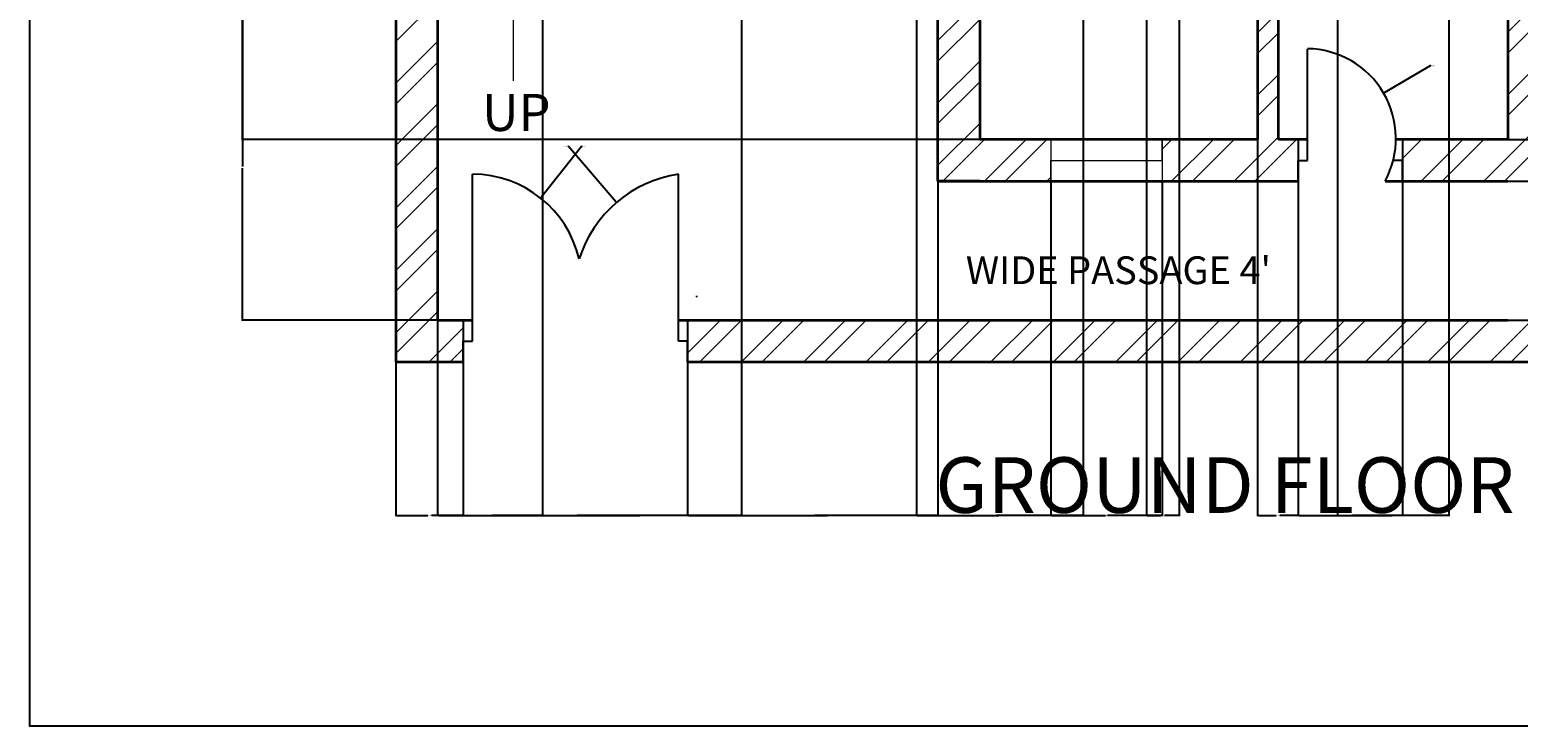
# Model space of a CAD drawing. Units: inches. Extents: x 1595 to 2135, y 460 to 2061.
# Tile 1 of 5: x 1595 to 1917, y 1320 to 1470. Entities that reach past the tile are written whole.
import ezdxf

# ---------------------------------------------------------------- set-up
doc = ezdxf.new("R2010")
doc.units = ezdxf.units.IN
for name, color, linetype, lineweight in [('A-ANNO-DIMS', 2, 'Continuous', 18), ('A-ANNO-SYMB', 7, 'Continuous', 18), ('A-ANNO-TTLB', 7, 'Continuous', 25), ('A-AREA-IDEN', 7, 'Continuous', 18), ('A-DOOR', 3, 'Continuous', 25), ('A-GLAZ', 4, 'Continuous', 18), ('A-WALL', 7, 'Continuous', 35)]:
    doc.layers.add(name, color=color, linetype=linetype, lineweight=lineweight)
doc.layers.add('A-WALL-PATT', color=143, linetype='Continuous', lineweight=13, true_color=0x7aafdf)
doc.styles.get("Standard").update_dxf_attribs({"font": 'arial.ttf'})
doc.dimstyles.get("Standard").update_dxf_attribs({"dimtxt": 0.18, "dimasz": 0.18, "dimexe": 0.18, "dimexo": 0.0625, "dimgap": 0.09, "dimtad": 0, "dimtih": 1, "dimtoh": 1, "dimdec": 4, "dimzin": 0, "dimdsep": 46, "dimtxsty": 'Standard', "dimcen": 0.09, "dimadec": 0, "dimazin": 0, "dimtfac": 1, "dimtdec": 4, "dimtofl": 0, "dimtmove": 0, "dimatfit": 3, "dimfxl": 1, "dimtolj": 1, "dimtzin": 0, "dimarcsym": 0})

# ---------------------------------------------------------------- blocks, each defined once
blk = doc.blocks.new('*D8')
at = {"layer": 'A-ANNO-DIMS', "color": 0, "lineweight": -2, "transparency": 16777216}
for p, q in [((1674.31, 1398.58), (1674.31, 1365.31)), ((1688.85, 1398.58), (1688.85, 1365.31)), ((1674.49, 1365.49), (1681.2, 1365.49)), ((1688.67, 1365.49), (1681.97, 1365.49))]:
    blk.add_line(p, q, dxfattribs=at)
at = {"layer": 'A-ANNO-DIMS', "color": 0, "transparency": 16777216}
for points in [[(1674.49, 1365.52), (1674.49, 1365.46), (1674.31, 1365.49)], [(1688.67, 1365.52), (1688.67, 1365.46), (1688.85, 1365.49)]]:
    blk.add_solid(points, dxfattribs=at)
at = {"layer": 'Defpoints', "color": 0, "transparency": 16777216}
for p in [(1674.31, 1398.64), (1688.85, 1398.64), (1688.85, 1365.49)]:
    blk.add_point(p, dxfattribs=at)
at = {"layer": 'A-ANNO-DIMS', "color": 0, "transparency": 16777216, "insert": (1681.58, 1365.49), "char_height": 0.18, "attachment_point": 5}
blk.add_mtext('\\A1;14.54', dxfattribs=at)
blk = doc.blocks.new('*D9')
at = {"layer": 'A-ANNO-DIMS', "color": 0, "lineweight": -2, "transparency": 16777216}
for p, q in [((1688.85, 1398.58), (1688.85, 1365.31)), ((1737.28, 1398.58), (1737.28, 1365.31)), ((1689.03, 1365.49), (1712.67, 1365.49)), ((1737.1, 1365.49), (1713.46, 1365.49))]:
    blk.add_line(p, q, dxfattribs=at)
at = {"layer": 'A-ANNO-DIMS', "color": 0, "transparency": 16777216}
for points in [[(1689.03, 1365.52), (1689.03, 1365.46), (1688.85, 1365.49)], [(1737.1, 1365.52), (1737.1, 1365.46), (1737.28, 1365.49)]]:
    blk.add_solid(points, dxfattribs=at)
at = {"layer": 'Defpoints', "color": 0, "transparency": 16777216}
for p in [(1688.85, 1398.64), (1737.28, 1398.64), (1737.28, 1365.49)]:
    blk.add_point(p, dxfattribs=at)
at = {"layer": 'A-ANNO-DIMS', "color": 0, "transparency": 16777216, "insert": (1713.06, 1365.49), "char_height": 0.18, "attachment_point": 5}
blk.add_mtext('\\A1;48.42', dxfattribs=at)
blk = doc.blocks.new('*D10')
at = {"layer": 'A-ANNO-DIMS', "color": 0, "lineweight": -2, "transparency": 16777216}
for p, q in [((1791.31, 1437.58), (1791.31, 1365.31)), ((1737.28, 1398.58), (1737.28, 1365.31)), ((1737.46, 1365.49), (1763.9, 1365.49)), ((1791.13, 1365.49), (1764.69, 1365.49))]:
    blk.add_line(p, q, dxfattribs=at)
at = {"layer": 'A-ANNO-DIMS', "color": 0, "transparency": 16777216}
for points in [[(1737.46, 1365.52), (1737.46, 1365.46), (1737.28, 1365.49)], [(1791.13, 1365.52), (1791.13, 1365.46), (1791.31, 1365.49)]]:
    blk.add_solid(points, dxfattribs=at)
at = {"layer": 'Defpoints', "color": 0, "transparency": 16777216}
for p in [(1791.31, 1437.64), (1737.28, 1398.64), (1791.31, 1365.49)]:
    blk.add_point(p, dxfattribs=at)
at = {"layer": 'A-ANNO-DIMS', "color": 0, "transparency": 16777216, "insert": (1764.29, 1365.49), "char_height": 0.18, "attachment_point": 5}
blk.add_mtext('\\A1;54.04', dxfattribs=at)
blk = doc.blocks.new('*D23')
at = {"layer": 'A-ANNO-DIMS', "color": 0, "lineweight": -2, "transparency": 16777216}
for p, q in [((1683.31, 1938.58), (1683.31, 1365.31)), ((1705.98, 1938.58), (1705.98, 1365.31)), ((1683.49, 1365.49), (1694.18, 1365.49)), ((1705.8, 1365.49), (1695.11, 1365.49))]:
    blk.add_line(p, q, dxfattribs=at)
at = {"layer": 'A-ANNO-DIMS', "color": 0, "transparency": 16777216}
for points in [[(1683.49, 1365.52), (1683.49, 1365.46), (1683.31, 1365.49)], [(1705.8, 1365.52), (1705.8, 1365.46), (1705.98, 1365.49)]]:
    blk.add_solid(points, dxfattribs=at)
at = {"layer": 'Defpoints', "color": 0, "transparency": 16777216}
for p in [(1683.31, 1938.64), (1705.98, 1938.64), (1705.98, 1365.49)]:
    blk.add_point(p, dxfattribs=at)
at = {"layer": 'A-ANNO-DIMS', "color": 0, "transparency": 16777216, "insert": (1694.64, 1365.49), "char_height": 0.18, "attachment_point": 5}
blk.add_mtext('\\A1;22.663', dxfattribs=at)
blk = doc.blocks.new('*D24')
at = {"layer": 'A-ANNO-DIMS', "color": 0, "lineweight": -2, "transparency": 16777216}
for p, q in [((1705.98, 1938.58), (1705.98, 1365.31)), ((1748.87, 1938.58), (1748.87, 1365.31)), ((1706.16, 1365.49), (1726.96, 1365.49)), ((1748.69, 1365.49), (1727.89, 1365.49))]:
    blk.add_line(p, q, dxfattribs=at)
at = {"layer": 'A-ANNO-DIMS', "color": 0, "transparency": 16777216}
for points in [[(1706.16, 1365.52), (1706.16, 1365.46), (1705.98, 1365.49)], [(1748.69, 1365.52), (1748.69, 1365.46), (1748.87, 1365.49)]]:
    blk.add_solid(points, dxfattribs=at)
at = {"layer": 'Defpoints', "color": 0, "transparency": 16777216}
for p in [(1705.98, 1938.64), (1748.87, 1938.64), (1748.87, 1365.49)]:
    blk.add_point(p, dxfattribs=at)
at = {"layer": 'A-ANNO-DIMS', "color": 0, "transparency": 16777216, "insert": (1727.42, 1365.49), "char_height": 0.18, "attachment_point": 5}
blk.add_mtext('\\A1;42.894', dxfattribs=at)
blk = doc.blocks.new('*D25')
at = {"layer": 'A-ANNO-DIMS', "color": 0, "lineweight": -2, "transparency": 16777216}
for p, q in [((1748.87, 1938.58), (1748.87, 1365.31)), ((1786.65, 1938.58), (1786.65, 1365.31)), ((1749.05, 1365.49), (1767.37, 1365.49)), ((1786.47, 1365.49), (1768.16, 1365.49))]:
    blk.add_line(p, q, dxfattribs=at)
at = {"layer": 'A-ANNO-DIMS', "color": 0, "transparency": 16777216}
for points in [[(1749.05, 1365.52), (1749.05, 1365.46), (1748.87, 1365.49)], [(1786.47, 1365.52), (1786.47, 1365.46), (1786.65, 1365.49)]]:
    blk.add_solid(points, dxfattribs=at)
at = {"layer": 'Defpoints', "color": 0, "transparency": 16777216}
for p in [(1748.87, 1938.64), (1786.65, 1938.64), (1786.65, 1365.49)]:
    blk.add_point(p, dxfattribs=at)
at = {"layer": 'A-ANNO-DIMS', "color": 0, "transparency": 16777216, "insert": (1767.76, 1365.49), "char_height": 0.18, "attachment_point": 5}
blk.add_mtext('\\A1;37.78', dxfattribs=at)
blk = doc.blocks.new('*D26')
at = {"layer": 'A-ANNO-DIMS', "color": 0, "lineweight": -2, "transparency": 16777216}
for p, q in [((1786.65, 1938.58), (1786.65, 1365.31)), ((1822.65, 1938.58), (1822.65, 1365.31)), ((1786.83, 1365.49), (1804.43, 1365.49)), ((1822.47, 1365.49), (1804.87, 1365.49))]:
    blk.add_line(p, q, dxfattribs=at)
at = {"layer": 'A-ANNO-DIMS', "color": 0, "transparency": 16777216}
for points in [[(1786.83, 1365.52), (1786.83, 1365.46), (1786.65, 1365.49)], [(1822.47, 1365.52), (1822.47, 1365.46), (1822.65, 1365.49)]]:
    blk.add_solid(points, dxfattribs=at)
at = {"layer": 'Defpoints', "color": 0, "transparency": 16777216}
for p in [(1786.65, 1938.64), (1822.65, 1938.64), (1822.65, 1365.49)]:
    blk.add_point(p, dxfattribs=at)
at = {"layer": 'A-ANNO-DIMS', "color": 0, "transparency": 16777216, "insert": (1804.65, 1365.49), "char_height": 0.18, "attachment_point": 5}
blk.add_mtext('\\A1;36', dxfattribs=at)
blk = doc.blocks.new('*D30')
at = {"layer": 'A-ANNO-DIMS', "color": 0, "lineweight": -2, "transparency": 16777216}
for p, q in [((1836.31, 1938.58), (1836.31, 1365.31)), ((1843.37, 1938.58), (1843.37, 1365.31)), ((1836.49, 1365.49), (1839.45, 1365.49)), ((1843.19, 1365.49), (1840.23, 1365.49))]:
    blk.add_line(p, q, dxfattribs=at)
at = {"layer": 'A-ANNO-DIMS', "color": 0, "transparency": 16777216}
for points in [[(1836.49, 1365.52), (1836.49, 1365.46), (1836.31, 1365.49)], [(1843.19, 1365.52), (1843.19, 1365.46), (1843.37, 1365.49)]]:
    blk.add_solid(points, dxfattribs=at)
at = {"layer": 'Defpoints', "color": 0, "transparency": 16777216}
for p in [(1836.31, 1938.64), (1843.37, 1938.64), (1843.37, 1365.49)]:
    blk.add_point(p, dxfattribs=at)
at = {"layer": 'A-ANNO-DIMS', "color": 0, "transparency": 16777216, "insert": (1839.84, 1365.49), "char_height": 0.18, "attachment_point": 5}
blk.add_mtext('\\A1;7.054', dxfattribs=at)
blk = doc.blocks.new('*D33')
at = {"layer": 'A-ANNO-DIMS', "color": 0, "lineweight": -2, "transparency": 16777216}
for p, q in [((1800.25, 1568.14), (1640.98, 1568.14)), ((1641.16, 1567.96), (1641.16, 1507.57)), ((1641.16, 1446.82), (1641.16, 1507.21)), ((1800.25, 1446.64), (1640.98, 1446.64))]:
    blk.add_line(p, q, dxfattribs=at)
at = {"layer": 'A-ANNO-DIMS', "color": 0, "transparency": 16777216}
for points in [[(1641.13, 1567.96), (1641.19, 1567.96), (1641.16, 1568.14)], [(1641.13, 1446.82), (1641.19, 1446.82), (1641.16, 1446.64)]]:
    blk.add_solid(points, dxfattribs=at)
at = {"layer": 'Defpoints', "color": 0, "transparency": 16777216}
for p in [(1641.16, 1568.14), (1800.31, 1568.14), (1800.31, 1446.64)]:
    blk.add_point(p, dxfattribs=at)
at = {"layer": 'A-ANNO-DIMS', "color": 0, "transparency": 16777216, "insert": (1641.16, 1507.39), "char_height": 0.18, "attachment_point": 5}
blk.add_mtext('\\A1;121.5', dxfattribs=at)
blk = doc.blocks.new('*D34')
at = {"layer": 'A-ANNO-DIMS', "color": 0, "lineweight": -2, "transparency": 16777216}
for p, q in [((1914.38, 1539.98), (2109.64, 1539.98)), ((2109.46, 1539.8), (2109.46, 1493.49)), ((2109.46, 1446.82), (2109.46, 1493.13)), ((1914.38, 1446.64), (2109.64, 1446.64))]:
    blk.add_line(p, q, dxfattribs=at)
at = {"layer": 'A-ANNO-DIMS', "color": 0, "transparency": 16777216}
for points in [[(2109.43, 1539.8), (2109.49, 1539.8), (2109.46, 1539.98)], [(2109.43, 1446.82), (2109.49, 1446.82), (2109.46, 1446.64)]]:
    blk.add_solid(points, dxfattribs=at)
at = {"layer": 'Defpoints', "color": 0, "transparency": 16777216}
for p in [(1914.31, 1539.98), (2109.46, 1539.98), (1914.31, 1446.64)]:
    blk.add_point(p, dxfattribs=at)
at = {"layer": 'A-ANNO-DIMS', "color": 0, "transparency": 16777216, "insert": (2109.46, 1493.31), "char_height": 0.18, "attachment_point": 5}
blk.add_mtext('\\A1;93.33', dxfattribs=at)
blk = doc.blocks.new('*D39')
at = {"layer": 'A-ANNO-DIMS', "color": 0, "lineweight": -2, "transparency": 16777216}
for p, q in [((1791.31, 1437.58), (1791.31, 1365.31)), ((1815.67, 1437.58), (1815.67, 1365.31)), ((1791.49, 1365.49), (1803.1, 1365.49)), ((1815.49, 1365.49), (1803.89, 1365.49))]:
    blk.add_line(p, q, dxfattribs=at)
at = {"layer": 'A-ANNO-DIMS', "color": 0, "transparency": 16777216}
for points in [[(1791.49, 1365.52), (1791.49, 1365.46), (1791.31, 1365.49)], [(1815.49, 1365.52), (1815.49, 1365.46), (1815.67, 1365.49)]]:
    blk.add_solid(points, dxfattribs=at)
at = {"layer": 'Defpoints', "color": 0, "transparency": 16777216}
for p in [(1791.31, 1437.64), (1815.67, 1437.64), (1815.67, 1365.49)]:
    blk.add_point(p, dxfattribs=at)
at = {"layer": 'A-ANNO-DIMS', "color": 0, "transparency": 16777216, "insert": (1803.49, 1365.49), "char_height": 0.18, "attachment_point": 5}
blk.add_mtext('\\A1;24.36', dxfattribs=at)
blk = doc.blocks.new('*D40')
at = {"layer": 'A-ANNO-DIMS', "color": 0, "lineweight": -2, "transparency": 16777216}
for p, q in [((1815.67, 1437.58), (1815.67, 1365.31)), ((1839.67, 1437.58), (1839.67, 1365.31)), ((1815.85, 1365.49), (1827.45, 1365.49)), ((1839.49, 1365.49), (1827.89, 1365.49))]:
    blk.add_line(p, q, dxfattribs=at)
at = {"layer": 'A-ANNO-DIMS', "color": 0, "transparency": 16777216}
for points in [[(1815.85, 1365.52), (1815.85, 1365.46), (1815.67, 1365.49)], [(1839.49, 1365.52), (1839.49, 1365.46), (1839.67, 1365.49)]]:
    blk.add_solid(points, dxfattribs=at)
at = {"layer": 'Defpoints', "color": 0, "transparency": 16777216}
for p in [(1815.67, 1437.64), (1839.67, 1437.64), (1839.67, 1365.49)]:
    blk.add_point(p, dxfattribs=at)
at = {"layer": 'A-ANNO-DIMS', "color": 0, "transparency": 16777216, "insert": (1827.67, 1365.49), "char_height": 0.18, "attachment_point": 5}
blk.add_mtext('\\A1;24', dxfattribs=at)
blk = doc.blocks.new('*D41')
at = {"layer": 'A-ANNO-DIMS', "color": 0, "lineweight": -2, "transparency": 16777216}
for p, q in [((1869.06, 1437.58), (1869.06, 1365.31)), ((1891.57, 1437.58), (1891.57, 1365.31)), ((1869.24, 1365.49), (1879.85, 1365.49)), ((1891.39, 1365.49), (1880.78, 1365.49))]:
    blk.add_line(p, q, dxfattribs=at)
at = {"layer": 'A-ANNO-DIMS', "color": 0, "transparency": 16777216}
for points in [[(1869.24, 1365.52), (1869.24, 1365.46), (1869.06, 1365.49)], [(1891.39, 1365.52), (1891.39, 1365.46), (1891.57, 1365.49)]]:
    blk.add_solid(points, dxfattribs=at)
at = {"layer": 'Defpoints', "color": 0, "transparency": 16777216}
for p in [(1869.06, 1437.64), (1891.57, 1437.64), (1891.57, 1365.49)]:
    blk.add_point(p, dxfattribs=at)
at = {"layer": 'A-ANNO-DIMS', "color": 0, "transparency": 16777216, "insert": (1880.32, 1365.49), "char_height": 0.18, "attachment_point": 5}
blk.add_mtext('\\A1;22.504', dxfattribs=at)
blk = doc.blocks.new('*D42')
at = {"layer": 'A-ANNO-DIMS', "color": 0, "lineweight": -2, "transparency": 16777216}
for p, q in [((1860.31, 1446.58), (1860.31, 1365.31)), ((1869.06, 1437.58), (1869.06, 1365.31)), ((1860.49, 1365.49), (1864.3, 1365.49)), ((1868.88, 1365.49), (1865.08, 1365.49))]:
    blk.add_line(p, q, dxfattribs=at)
at = {"layer": 'A-ANNO-DIMS', "color": 0, "transparency": 16777216}
for points in [[(1860.49, 1365.52), (1860.49, 1365.46), (1860.31, 1365.49)], [(1868.88, 1365.52), (1868.88, 1365.46), (1869.06, 1365.49)]]:
    blk.add_solid(points, dxfattribs=at)
at = {"layer": 'Defpoints', "color": 0, "transparency": 16777216}
for p in [(1860.31, 1446.64), (1869.06, 1437.64), (1869.06, 1365.49)]:
    blk.add_point(p, dxfattribs=at)
at = {"layer": 'A-ANNO-DIMS', "color": 0, "transparency": 16777216, "insert": (1864.69, 1365.49), "char_height": 0.18, "attachment_point": 5}
blk.add_mtext('\\A1;8.752', dxfattribs=at)
blk = doc.blocks.new('*D43')
at = {"layer": 'A-ANNO-DIMS', "color": 0, "lineweight": -2, "transparency": 16777216}
for p, q in [((1877.58, 1548.91), (1877.58, 1365.31)), ((1901.58, 1548.91), (1901.58, 1365.31)), ((1877.76, 1365.49), (1889.36, 1365.49)), ((1901.4, 1365.49), (1889.8, 1365.49))]:
    blk.add_line(p, q, dxfattribs=at)
at = {"layer": 'A-ANNO-DIMS', "color": 0, "transparency": 16777216}
for points in [[(1877.76, 1365.52), (1877.76, 1365.46), (1877.58, 1365.49)], [(1901.4, 1365.52), (1901.4, 1365.46), (1901.58, 1365.49)]]:
    blk.add_solid(points, dxfattribs=at)
at = {"layer": 'Defpoints', "color": 0, "transparency": 16777216}
for p in [(1877.58, 1548.98), (1901.58, 1548.98), (1901.58, 1365.49)]:
    blk.add_point(p, dxfattribs=at)
at = {"layer": 'A-ANNO-DIMS', "color": 0, "transparency": 16777216, "insert": (1889.58, 1365.49), "char_height": 0.18, "attachment_point": 5}
blk.add_mtext('\\A1;24', dxfattribs=at)
blk = doc.blocks.new('*D47')
at = {"layer": 'A-ANNO-DIMS', "color": 0, "lineweight": -2, "transparency": 16777216}
for p, q in [((1683.25, 1473.59), (1640.98, 1473.59)), ((1641.16, 1473.41), (1641.16, 1440.8)), ((1641.16, 1407.82), (1641.16, 1440.44)), ((1683.25, 1407.64), (1640.98, 1407.64))]:
    blk.add_line(p, q, dxfattribs=at)
at = {"layer": 'A-ANNO-DIMS', "color": 0, "transparency": 16777216}
for points in [[(1641.13, 1473.41), (1641.19, 1473.41), (1641.16, 1473.59)], [(1641.13, 1407.82), (1641.19, 1407.82), (1641.16, 1407.64)]]:
    blk.add_solid(points, dxfattribs=at)
at = {"layer": 'Defpoints', "color": 0, "transparency": 16777216}
for p in [(1641.16, 1473.59), (1683.31, 1473.59), (1683.31, 1407.64)]:
    blk.add_point(p, dxfattribs=at)
at = {"layer": 'A-ANNO-DIMS', "color": 0, "transparency": 16777216, "insert": (1641.16, 1440.62), "char_height": 0.18, "attachment_point": 5}
blk.add_mtext('\\A1;65.95', dxfattribs=at)
blk = doc.blocks.new('*D61')
at = {"layer": 'A-ANNO-DIMS', "color": 0, "lineweight": -2, "transparency": 16777216}
for p, q in [((1711.4, 1445.23), (1711.58, 1445.23)), ((1711.58, 1445.23), (1721.84, 1433.2)), ((1739.16, 1412.79), (1739.34, 1412.79)), ((1739.25, 1412.7), (1739.25, 1412.88))]:
    blk.add_line(p, q, dxfattribs=at)
at = {"layer": 'A-ANNO-DIMS', "color": 0, "transparency": 16777216}
blk.add_solid([(1721.86, 1433.22), (1721.81, 1433.18), (1721.95, 1433.06)], dxfattribs=at)
at = {"layer": 'Defpoints', "color": 0, "transparency": 16777216}
for p in [(1721.95, 1433.06), (1739.25, 1412.79)]:
    blk.add_point(p, dxfattribs=at)
at = {"layer": 'A-ANNO-DIMS', "color": 0, "transparency": 16777216, "insert": (1710.84, 1445.23), "char_height": 0.18, "attachment_point": 5}
blk.add_mtext('\\A1;R26.645', dxfattribs=at)
blk = doc.blocks.new('*D62')
at = {"layer": 'A-ANNO-DIMS', "color": 0, "lineweight": -2, "transparency": 16777216}
for p, q in [((1714.36, 1445.11), (1705.65, 1434.16)), ((1714.54, 1445.11), (1714.36, 1445.11)), ((1690.76, 1415.53), (1690.94, 1415.53)), ((1690.85, 1415.44), (1690.85, 1415.62))]:
    blk.add_line(p, q, dxfattribs=at)
at = {"layer": 'A-ANNO-DIMS', "color": 0, "transparency": 16777216}
blk.add_solid([(1705.63, 1434.18), (1705.68, 1434.14), (1705.54, 1434.02)], dxfattribs=at)
at = {"layer": 'Defpoints', "color": 0, "transparency": 16777216}
for p in [(1705.54, 1434.02), (1690.85, 1415.53)]:
    blk.add_point(p, dxfattribs=at)
at = {"layer": 'A-ANNO-DIMS', "color": 0, "transparency": 16777216, "insert": (1715, 1445.11), "char_height": 0.18, "attachment_point": 5}
blk.add_mtext('\\A1;R23.61', dxfattribs=at)
blk = doc.blocks.new('*D64')
at = {"layer": 'A-ANNO-DIMS', "color": 0, "lineweight": -2, "transparency": 16777216}
for p, q in [((1897.53, 1462.54), (1887.66, 1456.75)), ((1897.71, 1462.54), (1897.53, 1462.54)), ((1870.69, 1446.87), (1870.87, 1446.87)), ((1870.78, 1446.78), (1870.78, 1446.96))]:
    blk.add_line(p, q, dxfattribs=at)
at = {"layer": 'A-ANNO-DIMS', "color": 0, "transparency": 16777216}
blk.add_solid([(1887.64, 1456.78), (1887.67, 1456.73), (1887.5, 1456.66)], dxfattribs=at)
at = {"layer": 'Defpoints', "color": 0, "transparency": 16777216}
for p in [(1887.5, 1456.66), (1870.78, 1446.87)]:
    blk.add_point(p, dxfattribs=at)
at = {"layer": 'A-ANNO-DIMS', "color": 0, "transparency": 16777216, "insert": (1898.26, 1462.54), "char_height": 0.18, "attachment_point": 5}
blk.add_mtext('\\A1;R19.374', dxfattribs=at)

msp = doc.modelspace()

# ---------------------------------------------------------------- hatches: boundary and pattern name
at = {"layer": 'A-WALL-PATT'}
h = msp.add_hatch(dxfattribs=at)
h.set_pattern_fill('ANSI32', color=256)
h.paths.add_polyline_path([(2076.313, 2016.6421), (1674.313, 2016.6421), (1674.313, 1905.0731), (1683.313, 1905.0731), (1683.313, 1938.6421), (1705.9756, 1938.6421), (1705.9756, 1947.6421), (1683.313, 1947.6421), (1683.313, 2007.6421), (2067.313, 2007.6421), (2067.313, 1947.6421), (2046.0304, 1947.6421), (2046.0304, 1938.6421), (2067.313, 1938.6421), (2067.313, 1906.0373), (2076.313, 1906.0373), (2076.313, 1947.6421)])
h.paths.add_polyline_path([(1786.653, 1947.6421), (1748.8699, 1947.6421), (1748.8699, 1938.6421), (1786.653, 1938.6421), (1786.653, 1943.1421)], flags=17)
h.paths.add_polyline_path([(1843.367, 1943.1421), (1843.367, 1947.6421), (1822.653, 1947.6421), (1822.653, 1938.6421), (1827.313, 1938.6421), (1827.313, 1821.1082), (1836.313, 1821.1082), (1836.313, 1938.6421), (1843.367, 1938.6421)])
h.paths.add_polyline_path([(1928.933, 1943.1421), (1928.933, 1947.6421), (1875.313, 1947.6421), (1875.313, 1938.6421), (1914.313, 1938.6421), (1914.313, 1820.8892), (1923.313, 1820.8892), (1923.313, 1938.6421), (1928.933, 1938.6421)])
h.paths.add_polyline_path([(1997.1133, 1947.6421), (1964.933, 1947.6421), (1964.933, 1938.6421), (1997.1133, 1938.6421)], flags=17)
h.paths.add_polyline_path([(1974.313, 2007.6421), (1969.813, 2007.6421), (1969.813, 1947.6421), (1974.313, 1947.6421)], flags=17)
h.paths.add_polyline_path([(1780.813, 2007.6421), (1776.313, 2007.6421), (1776.313, 1947.6421), (1780.813, 1947.6421)], flags=17)
h.paths.add_polyline_path([(1683.313, 1845.0731), (1674.313, 1845.0731), (1674.313, 1734.209), (1683.313, 1734.209), (1683.313, 1773.6421), (1795.813, 1773.6421), (1836.313, 1773.6421), (1836.313, 1788.3627), (1831.813, 1788.3627), (1827.313, 1788.3627), (1827.313, 1782.6421), (1683.313, 1782.6421)])
h.paths.add_polyline_path([(2076.313, 1846.0373), (2067.313, 1846.0373), (2067.313, 1782.6421), (1923.313, 1782.6421), (1923.313, 1788.8802), (1918.813, 1788.8802), (1914.313, 1788.8802), (1914.313, 1773.6421), (2067.313, 1773.6421), (2067.313, 1710.6421), (2076.313, 1710.6421)])
h.paths.add_polyline_path([(1844.0531, 1859.9747), (1909.4596, 1859.9747), (1909.4596, 1882.3635), (1844.0531, 1882.3635)], flags=9)
h.paths.add_polyline_path([(1721.6058, 1827.3507), (1768.2143, 1827.3507), (1768.2143, 1849.7395), (1721.6058, 1849.7395)], flags=9)
h.paths.add_polyline_path([(1786.8661, 1359.2872), (1978.2276, 1359.2872), (1978.2276, 1384.0157), (1786.8661, 1384.0157)], flags=9)
h.paths.add_polyline_path([(1795.7228, 1412.0413), (1871.5904, 1412.0413), (1871.5904, 1424.4055), (1795.7228, 1424.4055)], flags=9)
h.paths.add_polyline_path([(1954.3634, 1526.3976), (2013.549, 1526.3976), (2013.549, 1548.7864), (1954.3634, 1548.7864)], flags=9)
h.paths.add_polyline_path([(1871.0596, 1490.4707), (1913.1292, 1490.4707), (1913.1292, 1512.8595), (1871.0596, 1512.8595)], flags=9)
h.paths.add_polyline_path([(1810.9452, 1510.8402), (1845.9343, 1510.8402), (1845.9343, 1533.229), (1810.9452, 1533.229)], flags=9)
h.paths.add_polyline_path([(1720.9117, 1692.9695), (1767.819, 1692.9695), (1767.819, 1715.3583), (1720.9117, 1715.3583)], flags=9)
h.paths.add_polyline_path([(1853.0254, 1698.4614), (1904.6966, 1698.4614), (1904.6966, 1720.8503), (1853.0254, 1720.8503)], flags=9)
h.paths.add_polyline_path([(1970.399, 1827.3507), (2017.0075, 1827.3507), (2017.0075, 1849.7395), (1970.399, 1849.7395)], flags=9)
h.paths.add_polyline_path([(1994.3418, 1955.5613), (2029.5928, 1955.5613), (2029.5928, 1977.9501), (1994.3418, 1977.9501)], flags=25)
h.paths.add_polyline_path([(1828.8665, 1964.6116), (1868.5173, 1964.6116), (1868.5173, 1987.0004), (1828.8665, 1987.0004)], flags=25)
h.paths.add_polyline_path([(1698.1483, 1960.8371), (1733.3994, 1960.8371), (1733.3994, 1983.2259), (1698.1483, 1983.2259)], flags=25)
h = msp.add_hatch(dxfattribs=at)
h.set_pattern_fill('ANSI32', color=256)
h.paths.add_polyline_path([(1683.313, 1641.6421), (1791.313, 1641.6421), (1791.313, 1634.7169), (1800.313, 1634.7169), (1800.313, 1650.6421), (1800.313, 1673.3054), (1795.813, 1673.3054), (1795.813, 1650.6421), (1683.313, 1650.6421), (1683.313, 1698.209), (1678.813, 1698.209), (1674.313, 1698.209), (1674.313, 1398.6421), (1688.853, 1398.6421), (1688.853, 1403.1421), (1688.853, 1407.6421), (1683.313, 1407.6421)])
h.paths.add_polyline_path([(1800.313, 1568.1421), (1827.2399, 1568.1421), (1827.2399, 1572.6421), (1827.2399, 1577.1421), (1800.313, 1577.1421), (1800.313, 1604.9472), (1795.813, 1604.9472), (1791.313, 1604.9472), (1791.313, 1437.6421), (1800.313, 1437.6421), (1815.6708, 1437.6421), (1815.6708, 1442.1421), (1815.6708, 1446.6421), (1800.313, 1446.6421)])
h.paths.add_polyline_path([(1877.5816, 1545.4284), (1877.5816, 1548.9761), (1864.813, 1548.9761), (1864.813, 1577.1421), (1852.144, 1577.1421), (1852.144, 1568.1421), (1860.313, 1568.1421), (1860.313, 1446.6421), (1839.6708, 1446.6421), (1839.6708, 1437.6421), (1869.0647, 1437.6421), (1869.0647, 1442.1421), (1869.0647, 1446.6421), (1864.813, 1446.6421), (1864.813, 1539.9761), (1877.5816, 1539.9761), (1877.5816, 1541.8808)])
h.paths.add_polyline_path([(1923.313, 1568.1421), (1936.607, 1568.1421), (1936.607, 1577.1421), (1914.313, 1577.1421), (1914.313, 1548.9761), (1901.5816, 1548.9761), (1901.5816, 1539.9761), (1914.313, 1539.9761), (1914.313, 1446.6421), (1891.5684, 1446.6421), (1891.5684, 1437.6421), (1914.313, 1437.6421), (1923.313, 1437.6421)])
h.paths.add_polyline_path([(2067.313, 1577.1421), (2003.1294, 1577.1421), (2003.1294, 1568.1421), (2067.313, 1568.1421)])
h.paths.add_polyline_path([(2076.313, 1650.6421), (2067.313, 1650.6421), (2067.313, 1504.2035), (2076.313, 1504.2035)])
h.paths.add_polyline_path([(2076.313, 1444.2035), (2071.813, 1444.2035), (2067.313, 1444.2035), (2067.313, 1407.6421), (1923.313, 1407.6421), (1918.813, 1407.6421), (1914.313, 1407.6421), (1737.2767, 1407.6421), (1737.2767, 1398.6421), (2076.313, 1398.6421)])

# ---------------------------------------------------------------- linework, layer by layer
at = {"layer": 'A-ANNO-SYMB'}
msp.add_line((1699.6809, 1459.3163), (1699.6809, 1624.3644), dxfattribs=at)
at = {"layer": 'A-ANNO-TTLB'}
msp.add_lwpolyline([(1595.2754, 2061.0707), (2134.6206, 2061.0707), (2134.6206, 1319.9937), (1595.2754, 1319.9937)], close=True, dxfattribs=at)
at = {"layer": 'A-DOOR'}
for p, q in [((1871.0647, 1442.1421), (1871.0647, 1466.1421)), ((1869.0647, 1446.6421), (1869.0647, 1437.6421)), ((1891.5684, 1446.6421), (1891.5684, 1437.6421)), ((1869.0647, 1437.6421), (1869.0647, 1442.1421)), ((1869.0647, 1442.1421), (1871.0647, 1442.1421)), ((1891.5684, 1442.1421), (1889.5684, 1442.1421)), ((1891.5684, 1437.6421), (1891.5684, 1442.1421)), ((1690.853, 1403.1421), (1690.853, 1439.1421)), ((1735.2767, 1403.1421), (1735.2767, 1439.1421)), ((1914.313, 1437.6421), (1923.313, 1437.6421)), ((1688.853, 1407.6421), (1688.853, 1398.6421)), ((1737.2767, 1407.6421), (1737.2767, 1398.6421)), ((1914.313, 1407.6421), (1923.313, 1407.6421)), ((1688.853, 1398.6421), (1688.853, 1403.1421)), ((1688.853, 1403.1421), (1690.853, 1403.1421)), ((1737.2767, 1403.1421), (1735.2767, 1403.1421)), ((1737.2767, 1398.6421), (1737.2767, 1403.1421))]:
    msp.add_line(p, q, dxfattribs=at)
for centre, radius, start, end in [((1870.7812, 1446.8735), 19.3738, 331.543603, 89.16173), ((1690.853, 1415.5331), 23.609, 13.048368, 90), ((1739.2462, 1412.7945), 26.6449, 98.567748, 162.372357)]:
    msp.add_arc(centre, radius, start, end, dxfattribs=at)
at = {"layer": 'A-GLAZ'}
for p, q in [((1815.6708, 1446.6421), (1815.6708, 1437.6421)), ((1839.6708, 1442.1421), (1839.6708, 1446.6421)), ((1839.6708, 1446.6421), (1839.6708, 1437.6421)), ((1815.6708, 1437.6421), (1815.6708, 1442.1421)), ((1815.6708, 1442.1421), (1839.6708, 1442.1421))]:
    msp.add_line(p, q, dxfattribs=at)
at = {"layer": 'A-WALL'}
for p, q in [((1674.313, 2016.6421), (1674.313, 1398.6421)), ((1683.313, 1641.6421), (1683.313, 1407.6421)), ((1791.313, 1437.6421), (1791.313, 1605.8316)), ((1800.313, 1568.1421), (1800.313, 1446.6421)), ((1860.313, 1568.1421), (1860.313, 1446.6421)), ((1864.813, 1446.6421), (1864.813, 1539.9761)), ((1914.313, 1539.9761), (1914.313, 1446.6421)), ((1860.313, 1446.6421), (1800.313, 1446.6421)), ((1871.0647, 1446.6421), (1864.813, 1446.6421)), ((1914.313, 1446.6421), (1890.1537, 1446.6421)), ((1791.313, 1437.6421), (1869.0647, 1437.6421)), ((1800.313, 1437.6421), (1791.313, 1437.6421)), ((1887.8143, 1437.6421), (1914.313, 1437.6421)), ((1914.313, 1437.6421), (1914.313, 1437.6421)), ((1683.313, 1407.6421), (1690.853, 1407.6421)), ((1735.2767, 1407.6421), (1914.313, 1407.6421)), ((1674.313, 1398.6421), (1688.853, 1398.6421)), ((1737.2767, 1398.6421), (2076.313, 1398.6421))]:
    msp.add_line(p, q, dxfattribs=at)

# ---------------------------------------------------------------- texts
at = {"layer": 'A-ANNO-SYMB', "insert": (1692.9175, 1456.4822), "char_height": 8, "attachment_point": 1}
msp.add_mtext_dynamic_manual_height_columns('UP', width=27.1977, gutter_width=12.5, heights=[0], dxfattribs=at)
at = {"layer": 'A-ANNO-TTLB', "insert": (1790.7583, 1378.0525), "char_height": 12, "attachment_point": 1, "line_spacing_factor": 2.88}
msp.add_mtext_dynamic_manual_height_columns('GROUND FLOOR PLAN ', width=392.566159, gutter_width=12.5, heights=[0], dxfattribs=at)
at = {"layer": 'A-AREA-IDEN', "insert": (1797.3251, 1421.4199), "char_height": 6, "attachment_point": 1}
msp.add_mtext_dynamic_manual_height_columns("WIDE PASSAGE 4'", width=89.543375, gutter_width=12.5, heights=[0], dxfattribs=at)

# ---------------------------------------------------------------- dimensions: what is measured, and where the dimension line sits
at = {"layer": 'A-ANNO-DIMS'}
for base, p1, p2, override, picture, middle in [((1705.9756, 1365.4921), (1683.313, 1938.6421), (1705.9756, 1938.6421), {"dimdec": 3, "dimlfac": 1, "dimrnd": 0, "dimzin": 0, "dimdsep": 46, "dimlunit": 2}, '*D23', (1694.6443, 1365.4921)), ((1748.8699, 1365.4921), (1705.9756, 1938.6421), (1748.8699, 1938.6421), {"dimdec": 3, "dimlfac": 1, "dimrnd": 0, "dimzin": 0, "dimdsep": 46, "dimlunit": 2}, '*D24', (1727.4227, 1365.4921)), ((1786.653, 1365.4921), (1748.8699, 1938.6421), (1786.653, 1938.6421), {"dimdec": 2, "dimlfac": 1, "dimrnd": 0, "dimzin": 0, "dimdsep": 46, "dimlunit": 2}, '*D25', (1767.7614, 1365.4921)), ((1822.653, 1365.4921), (1786.653, 1938.6421), (1822.653, 1938.6421), {"dimdec": 0, "dimlfac": 1, "dimrnd": 0, "dimzin": 0, "dimdsep": 46, "dimlunit": 2}, '*D26', (1804.653, 1365.4921)), ((1843.367, 1365.4921), (1836.313, 1938.6421), (1843.367, 1938.6421), {"dimdec": 3, "dimlfac": 1, "dimrnd": 0, "dimzin": 0, "dimdsep": 46, "dimlunit": 2}, '*D30', (1839.84, 1365.4921)), ((1901.5816, 1365.4921), (1877.5816, 1548.9761), (1901.5816, 1548.9761), {"dimdec": 0, "dimlfac": 1, "dimrnd": 0, "dimzin": 0, "dimdsep": 46, "dimlunit": 2}, '*D43', (1889.5816, 1365.4921)), ((1869.0647, 1365.4921), (1860.313, 1446.6421), (1869.0647, 1437.6421), {"dimdec": 3, "dimlfac": 1, "dimrnd": 0, "dimzin": 0, "dimdsep": 46, "dimlunit": 2}, '*D42', (1864.6888, 1365.4921)), ((1791.313, 1365.4921), (1737.2767, 1398.6421), (1791.313, 1437.6421), {"dimdec": 2, "dimlfac": 1, "dimrnd": 0, "dimzin": 0, "dimdsep": 46, "dimlunit": 2}, '*D10', (1764.2949, 1365.4921)), ((1815.6708, 1365.4921), (1791.313, 1437.6421), (1815.6708, 1437.6421), {"dimdec": 2, "dimlfac": 1, "dimrnd": 0, "dimzin": 0, "dimdsep": 46, "dimlunit": 2}, '*D39', (1803.4919, 1365.4921)), ((1839.6708, 1365.4921), (1815.6708, 1437.6421), (1839.6708, 1437.6421), {"dimdec": 0, "dimlfac": 1, "dimrnd": 0, "dimzin": 0, "dimdsep": 46, "dimlunit": 2}, '*D40', (1827.6708, 1365.4921)), ((1891.5684, 1365.4921), (1869.0647, 1437.6421), (1891.5684, 1437.6421), {"dimdec": 3, "dimlfac": 1, "dimrnd": 0, "dimzin": 0, "dimdsep": 46, "dimlunit": 2}, '*D41', (1880.3165, 1365.4921)), ((1688.853, 1365.4921), (1674.313, 1398.6421), (1688.853, 1398.6421), {"dimdec": 2, "dimlfac": 1, "dimrnd": 0, "dimzin": 0, "dimdsep": 46, "dimlunit": 2}, '*D8', (1681.583, 1365.4921)), ((1737.2767, 1365.4921), (1688.853, 1398.6421), (1737.2767, 1398.6421), {"dimdec": 2, "dimlfac": 1, "dimrnd": 0, "dimzin": 0, "dimdsep": 46, "dimlunit": 2}, '*D9', (1713.0649, 1365.4921))]:
    dim = msp.add_linear_dim(base=base, p1=p1, p2=p2, dimstyle='Standard', override=override, dxfattribs=at)
    dim.commit()
    dim.dimension.update_dxf_attribs({"geometry": picture, "text_midpoint": middle})
for base, p1, p2, override, picture, middle in [((1641.163, 1568.1421), (1800.313, 1446.6421), (1800.313, 1568.1421), {"dimdec": 1, "dimlfac": 1, "dimrnd": 0, "dimzin": 0, "dimdsep": 46, "dimlunit": 2}, '*D33', (1641.163, 1507.3921)), ((2109.463, 1539.9761), (1914.313, 1446.6421), (1914.313, 1539.9761), {"dimdec": 2, "dimlfac": 1, "dimrnd": 0, "dimzin": 0, "dimdsep": 46, "dimlunit": 2}, '*D34', (2109.463, 1493.3091)), ((1641.163, 1473.5918), (1683.313, 1407.6421), (1683.313, 1473.5918), {"dimdec": 2, "dimlfac": 1, "dimrnd": 0, "dimzin": 0, "dimdsep": 46, "dimlunit": 2}, '*D47', (1641.163, 1440.6169))]:
    dim = msp.add_linear_dim(base=base, p1=p1, p2=p2, angle=90, dimstyle='Standard', override=override, dxfattribs=at)
    dim.commit()
    dim.dimension.update_dxf_attribs({"geometry": picture, "text_midpoint": middle})
for center, mpoint, override, picture, middle in [((1870.7812, 1446.8735), (1887.4999, 1456.6629), {"dimdec": 3, "dimlfac": 1, "dimrnd": 0, "dimzin": 0, "dimdsep": 46, "dimlunit": 2}, '*D64', (1898.2604, 1462.5366)), ((1690.853, 1415.5331), (1705.542, 1434.016), {"dimdec": 2, "dimlfac": 1, "dimrnd": 0, "dimzin": 0, "dimdsep": 46, "dimlunit": 2}, '*D62', (1714.9978, 1445.1057)), ((1739.2462, 1412.7945), (1721.9519, 1433.0641), {"dimdec": 3, "dimlfac": 1, "dimrnd": 0, "dimzin": 0, "dimdsep": 46, "dimlunit": 2}, '*D61', (1710.8449, 1445.2259))]:
    dim = msp.add_radius_dim(center=center, mpoint=mpoint, dimstyle='Standard', override=override, dxfattribs=at)
    dim.commit()
    dim.dimension.update_dxf_attribs({"geometry": picture, "text_midpoint": middle, "dimtype": 164})

doc.saveas('drawing.dxf')
